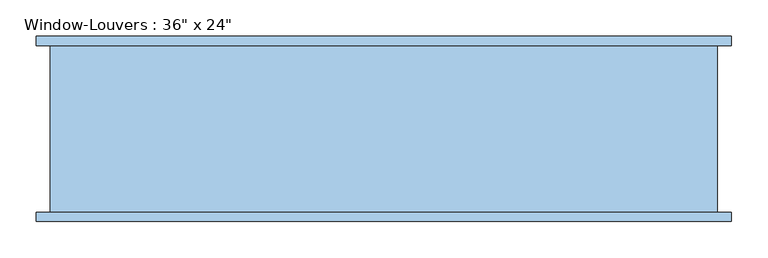
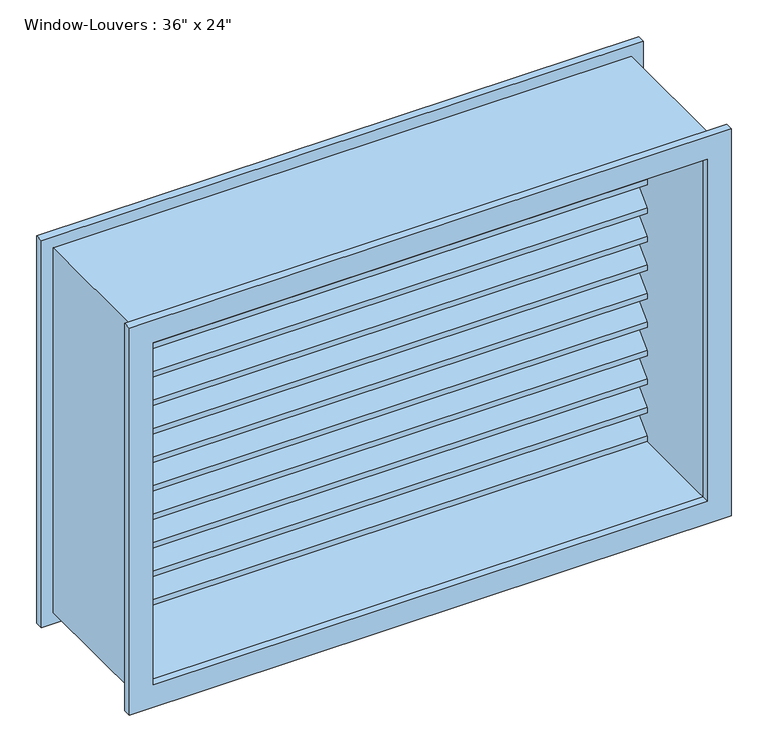
"""IFC4 building model written with IfcOpenShell, lengths in millimetres: window geometry."""

from ifc_helpers import new_model, si_unit, frame, origin, place, context, project, spatial, polyline, outline, extrude, source, transform, mapped, element, save


def window_a18e4be4(model_context):
    return source(origin(), model_context, "Body", "SweptSolid", [
        extrude(outline(polyline([(107.95, 1419.1754778), (107.95, 1410.1952217), (69.85, 1448.2952217), (31.75, 1410.1952217), (31.75, 1419.1754778), (69.85, 1457.2754778), (107.95, 1419.1754778)])), frame((-438.15, 0.0, 0.0), z_axis=(1.0, 0.0, 0.0), x_axis=(0.0, 1.0, 0.0)), (0.0, 0.0, 1.0), 876.3),
        extrude(outline(polyline([(107.95, 1371.5009557), (107.95, 1362.5206995), (69.85, 1400.6206995), (31.75, 1362.5206995), (31.75, 1371.5009557), (69.85, 1409.6009557), (107.95, 1371.5009557)])), frame((-438.15, 0.0, 0.0), z_axis=(1.0, 0.0, 0.0), x_axis=(0.0, 1.0, 0.0)), (0.0, 0.0, 1.0), 876.3),
        extrude(outline(polyline([(107.95, 1323.8264335), (107.95, 1314.8461774), (69.85, 1352.9461774), (31.75, 1314.8461774), (31.75, 1323.8264335), (69.85, 1361.9264335), (107.95, 1323.8264335)])), frame((-438.15, 0.0, 0.0), z_axis=(1.0, 0.0, 0.0), x_axis=(0.0, 1.0, 0.0)), (0.0, 0.0, 1.0), 876.3),
        extrude(outline(polyline([(107.95, 1276.1519113), (107.95, 1267.1716552), (69.85, 1305.2716552), (31.75, 1267.1716552), (31.75, 1276.1519113), (69.85, 1314.2519113), (107.95, 1276.1519113)])), frame((-438.15, 0.0, 0.0), z_axis=(1.0, 0.0, 0.0), x_axis=(0.0, 1.0, 0.0)), (0.0, 0.0, 1.0), 876.3),
        extrude(outline(polyline([(107.95, 1228.4773891), (107.95, 1219.497133), (69.85, 1257.597133), (31.75, 1219.497133), (31.75, 1228.4773891), (69.85, 1266.5773891), (107.95, 1228.4773891)])), frame((-438.15, 0.0, 0.0), z_axis=(1.0, 0.0, 0.0), x_axis=(0.0, 1.0, 0.0)), (0.0, 0.0, 1.0), 876.3),
        extrude(outline(polyline([(107.95, 1180.802867), (107.95, 1171.8226109), (69.85, 1209.9226109), (31.75, 1171.8226109), (31.75, 1180.802867), (69.85, 1218.902867), (107.95, 1180.802867)])), frame((-438.15, 0.0, 0.0), z_axis=(1.0, 0.0, 0.0), x_axis=(0.0, 1.0, 0.0)), (0.0, 0.0, 1.0), 876.3),
        extrude(outline(polyline([(107.95, 1133.1283448), (107.95, 1124.1480887), (69.85, 1162.2480887), (31.75, 1124.1480887), (31.75, 1133.1283448), (69.85, 1171.2283448), (107.95, 1133.1283448)])), frame((-438.15, 0.0, 0.0), z_axis=(1.0, 0.0, 0.0), x_axis=(0.0, 1.0, 0.0)), (0.0, 0.0, 1.0), 876.3),
        extrude(outline(polyline([(107.95, 1085.4538226), (107.95, 1076.4735665), (69.85, 1114.5735665), (31.75, 1076.4735665), (31.75, 1085.4538226), (69.85, 1123.5538226), (107.95, 1085.4538226)])), frame((-438.15, 0.0, 0.0), z_axis=(1.0, 0.0, 0.0), x_axis=(0.0, 1.0, 0.0)), (0.0, 0.0, 1.0), 876.3),
        extrude(outline(polyline([(107.95, 1037.7793005), (107.95, 1028.7990443), (69.85, 1066.8990443), (31.75, 1028.7990443), (31.75, 1037.7793005), (69.85, 1075.8793005), (107.95, 1037.7793005)])), frame((-438.15, 0.0, 0.0), z_axis=(1.0, 0.0, 0.0), x_axis=(0.0, 1.0, 0.0)), (0.0, 0.0, 1.0), 876.3),
        extrude(outline(polyline([(107.95, 990.1047783), (107.95, 981.1245222), (69.85, 1019.2245222), (31.75, 981.1245222), (31.75, 990.1047783), (69.85, 1028.2047783), (107.95, 990.1047783)])), frame((-438.15, 0.0, 0.0), z_axis=(1.0, 0.0, 0.0), x_axis=(0.0, 1.0, 0.0)), (0.0, 0.0, 1.0), 876.3),
        extrude(outline(polyline([(107.95, 1466.85), (107.95, 1457.8697439), (69.85, 1495.9697439), (31.75, 1457.8697439), (31.75, 1466.85), (69.85, 1504.95), (107.95, 1466.85)])), frame((-438.15, 0.0, 0.0), z_axis=(1.0, 0.0, 0.0), x_axis=(0.0, 1.0, 0.0)), (0.0, 0.0, 1.0), 876.3),
        extrude(outline(polyline([(107.95, 942.4302561), (107.95, 933.45), (69.85, 971.55), (31.75, 933.45), (31.75, 942.4302561), (69.85, 980.5302561), (107.95, 942.4302561)])), frame((-438.15, 0.0, 0.0), z_axis=(1.0, 0.0, 0.0), x_axis=(0.0, 1.0, 0.0)), (0.0, 0.0, 1.0), 876.3),
        extrude(outline(polyline([(1524.0, 457.2), (1524.0, -457.2), (914.4, -457.2), (914.4, 457.2), (1524.0, 457.2)]), holes=[polyline([(1504.95, 438.15), (933.45, 438.15), (933.45, -438.15), (1504.95, -438.15), (1504.95, 438.15)])]), frame((0.0, -120.65, 0.0), z_axis=(0.0, 1.0, 0.0), x_axis=(0.0, 0.0, 1.0)), (0.0, 0.0, 1.0), 228.6),
        extrude(outline(polyline([(1543.05, 476.25), (1543.05, -476.25), (895.35, -476.25), (895.35, 476.25), (1543.05, 476.25)]), holes=[polyline([(1504.95, 438.15), (933.45, 438.15), (933.45, -438.15), (1504.95, -438.15), (1504.95, 438.15)])]), frame((0.0, -133.35, 0.0), z_axis=(0.0, 1.0, 0.0), x_axis=(0.0, 0.0, 1.0)), (0.0, 0.0, 1.0), 12.7),
        extrude(outline(polyline([(1543.05, -476.25), (895.35, -476.25), (895.35, 476.25), (1543.05, 476.25), (1543.05, -476.25)]), holes=[polyline([(1504.95, -438.15), (1504.95, 438.15), (933.45, 438.15), (933.45, -438.15), (1504.95, -438.15)])]), frame((0.0, 107.95, 0.0), z_axis=(0.0, 1.0, 0.0), x_axis=(0.0, 0.0, 1.0)), (0.0, 0.0, 1.0), 12.7),
    ])


if __name__ == "__main__":
    model = new_model("IFC4")
    model_context = context("Model", 3, world=origin())
    ifc_project = project(units=[si_unit("LENGTHUNIT", "METRE", prefix="MILLI")], contexts=[model_context])
    site = spatial("IfcSite", under=ifc_project)
    building = spatial("IfcBuilding", under=site)
    placement = place(None, origin())
    window_shape = window_a18e4be4(model_context)
    element("IfcWindow", 1, ObjectType="Window-Louvers : 36\" x 24\"", at=placement, inside=building, context=model_context, shape_type="MappedRepresentation", body=[
        mapped(window_shape, transform((0.0, 0.0, 0.0), x_axis=(1.0, 0.0, 0.0), y_axis=(0.0, 1.0, 0.0), z_axis=(0.0, 0.0, 1.0))),
    ])
    save(model, "model.ifc")

# Revit data of these elements
# Type "Window-Louvers : 36\" x 24\""
#   Type Mark = "18"
#   Construction Type Id = "GSP4R"
#   Assembly Code = "B20"
#   Analytic Construction = "1/8 in Pilkington single glazing"
#   Visual Light Transmittance = 0.9
#   Thermal Resistance (R) = 1.53941 (h·ft²·°F)/BTU
#   Solar Heat Gain Coefficient = 0.78
#   Max Height = 1' - 11.74264"
#   Height = 2' - 0"
#   Heat Transfer Coefficient (U) = 0.6496 BTU/(h·ft²·°F)
#   Blade Width [instance default] = 2' - 10 1/2"
#   Blade Vertical Thickness = 0' - 0.35355"
#   Blade Thickness = 0' - 0 1/4"
#   Blade Spacing = 0' - 1 1/2"
#   Blade Height = 0' - 1.85355"
#   Blade Depth = 0' - 3"
#   Blade Angle = 45.00°
#   Default Sill Height = 3' - 0"
#   Trim Projection_Exterior = 0' - 0 1/2"
#   Trim Projection_Interior = 0' - 0 1/2"
#   Trim Width_Exterior = 0' - 1 1/2"
#   Trim Width_Interior = 0' - 1 1/2"
#   Width = 3' - 0"
#   Max Blade Count = 12
#   Define Thermal Properties by = 1
#   Blade Count = 12
#   Frame Material = Birch
#   Louver Material = Birch
#   Trim Exterior Material = Birch
#   Trim Interior Material = Birch
#   Wall Closure = (empty or 0)
# Element 1 (IfcWindow, "Window-Louvers : 36\" x 24\"")
#   Materials on its faces: "Birch"
# Materials
#   "Birch": class "Wood", colour RGB 224 178 126, transparency 0, Description = "Betula Alleghaniensis", Cost = 0
